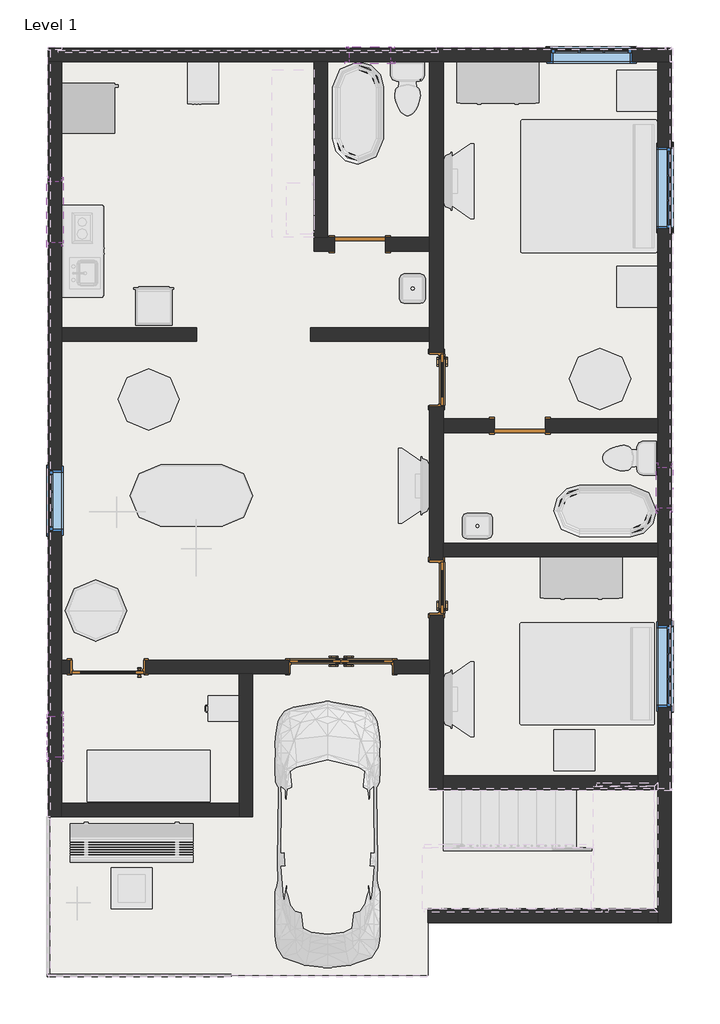
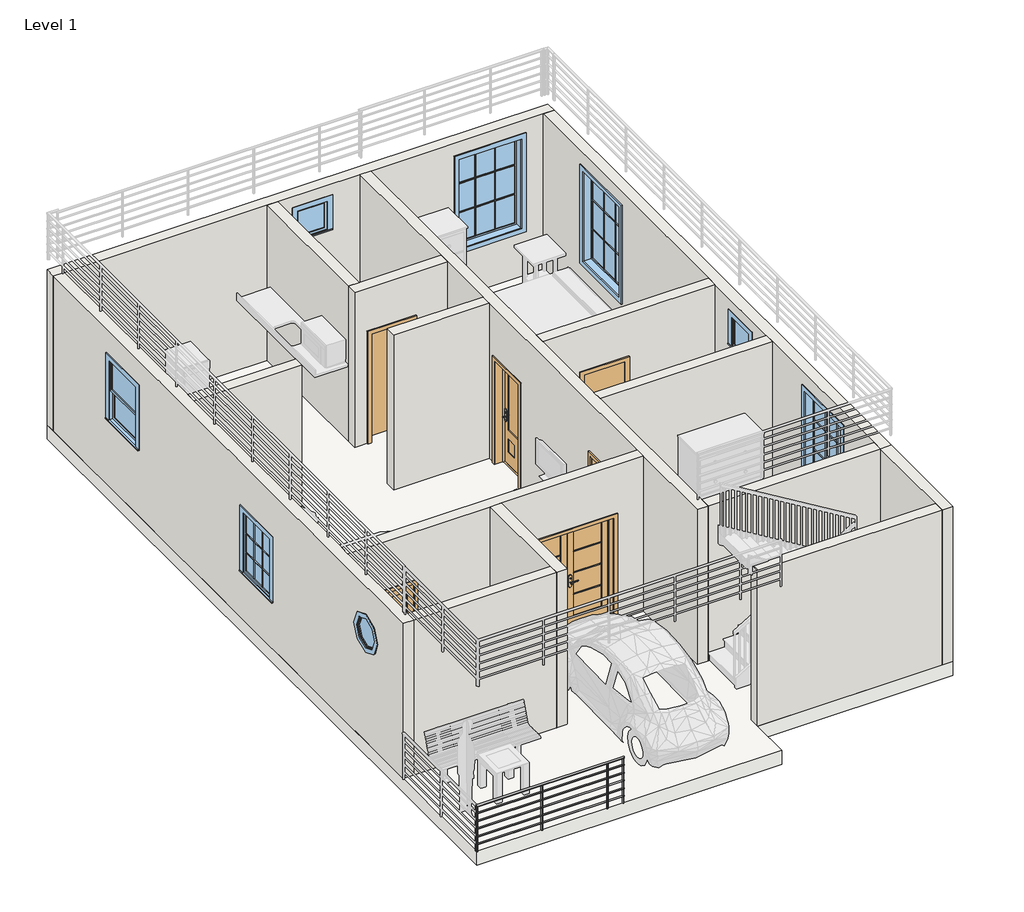
# One storey, part 1 of 4: 15 walls, 8 windows, 6 doors, 1 railing, 1 slab.
"""IFC4 building model written with IfcOpenShell, lengths in millimetres."""

from ifc_helpers import new_model, si_unit, point, frame, frame_2d, origin, origin_with_axes, place, context, project, spatial, polyline, circle_curve, trimmed, segment, composite_curve, outline, extrude, faceted_brep, transform, mapped, element, save
from ifc_brep_helpers import plane_surface, revolved_surface, advanced_brep
from components import door_ad59dcae, door_41326d50, door_b03bd389, door_f3911013, door_4314e8ec, window_29c06734, window_5a4e61ec, window_31198920, window_3923817a, window_e41d21a6

model = new_model("IFC4")

# Units and contexts
model_context = context("Model", 3, world=origin())
ifc_project = project(units=[si_unit("LENGTHUNIT", "METRE", prefix="MILLI")], contexts=[model_context])

# Site, building, storey
site = spatial("IfcSite", under=ifc_project)
building = spatial("IfcBuilding", under=site)
storey = spatial("IfcBuildingStorey", under=building, Name="Level 1", Elevation=0.0)

# Doors
placement = place(None, origin())
door_shape = door_ad59dcae(model_context)
element("IfcDoor", 1, ObjectType="30\" x 80\"", at=placement, inside=storey, context=model_context, shape_type="MappedRepresentation", body=[
    mapped(door_shape, transform((-8628.2639568, 7069.0342758, 0.0), x_axis=(0.0, -1.0, 0.0), y_axis=(1.0, 0.0, 0.0), z_axis=(0.0, 0.0, 1.0))),
])
door_2_shape = door_41326d50(model_context)
element("IfcDoor", 2, ObjectType="30\" x 80\"", at=placement, inside=storey, context=model_context, shape_type="MappedRepresentation", body=[
    mapped(door_2_shape, transform((-8628.2639568, 10167.8342758, 0.0), x_axis=(0.0, 1.0, 0.0), y_axis=(-1.0, 0.0, 0.0), z_axis=(0.0, 0.0, 1.0))),
])
door_3_shape = door_b03bd389(model_context)
element("IfcDoor", 3, ObjectType="Door-Exterior-Double-Full Glass-Wood_Clad : 60\" x 80\"", at=placement, inside=storey, context=model_context, shape_type="MappedRepresentation", body=[
    mapped(door_3_shape, transform((-10053.8389568, 5891.1092758, 0.0), x_axis=(1.0, 0.0, 0.0), y_axis=(0.0, 1.0, 0.0), z_axis=(0.0, 0.0, 1.0))),
])
door_4_shape = door_f3911013(model_context)
element("IfcDoor", 4, ObjectType="Door-Interior-Single-Full Glass-Wood : 42\" x 80\"", at=placement, inside=storey, context=model_context, shape_type="MappedRepresentation", body=[
    mapped(door_4_shape, transform((-13533.6389568, 5884.7592758, 0.0), x_axis=(-1.0, 0.0, 0.0), y_axis=(0.0, -1.0, 0.0), z_axis=(0.0, 0.0, 1.0))),
])
door_5_shape = door_4314e8ec(model_context)
element("IfcDoor", 5, ObjectType="Single-Flush : 30\" x 84\"", at=placement, inside=storey, context=model_context, shape_type="MappedRepresentation", body=[
    mapped(door_5_shape, transform((-9774.4389568, 12187.1342758, 0.0), x_axis=(-1.0, 0.0, 0.0), y_axis=(0.0, -1.0, 0.0), z_axis=(0.0, 0.0, 1.0))),
])
element("IfcDoor", 6, ObjectType="Single-Flush : 30\" x 84\"", at=placement, inside=storey, context=model_context, shape_type="MappedRepresentation", body=[
    mapped(door_5_shape, transform((-7386.8389568, 9482.0342758, 0.0), x_axis=(1.0, 0.0, 0.0), y_axis=(0.0, 1.0, 0.0), z_axis=(0.0, 0.0, 1.0))),
])

# Railing
element("IfcRailing", 7, ObjectType="Handrail - Pipe", at=placement, inside=storey, context=model_context, shape_type="SweptSolid", body=[
    extrude(outline(composite_curve([segment(trimmed(circle_curve(frame_2d((1290.5342758, 895.35)), 19.05), [point((1271.4842758, 895.35))], [point((1309.5842758, 895.35))], False, "CARTESIAN"), True, "CONTINUOUS"), segment(trimmed(circle_curve(frame_2d((1290.5342758, 895.35)), 19.05), [point((1309.5842758, 895.35))], [point((1271.4842758, 895.35))], False, "CARTESIAN"), True, "CONTINUOUS")], self_intersect=False)), frame((-14435.3389568, 0.0, 0.0), z_axis=(1.0, 0.0, 0.0), x_axis=(0.0, 1.0, 0.0)), (0.0, 0.0, 1.0), 2743.2),
    extrude(outline(composite_curve([segment(trimmed(circle_curve(frame_2d((1290.5342758, 749.3)), 12.7), [point((1303.2342758, 749.3))], [point((1277.8342758, 749.3))], False, "CARTESIAN"), True, "CONTINUOUS"), segment(trimmed(circle_curve(frame_2d((1290.5342758, 749.3)), 12.7), [point((1277.8342758, 749.3))], [point((1303.2342758, 749.3))], False, "CARTESIAN"), True, "CONTINUOUS")], self_intersect=False)), frame((-14435.3389568, 0.0, 0.0), z_axis=(1.0, 0.0, 0.0), x_axis=(0.0, 1.0, 0.0)), (0.0, 0.0, 1.0), 2743.2),
    extrude(outline(composite_curve([segment(trimmed(circle_curve(frame_2d((1290.5342758, 596.9)), 12.7), [point((1303.2342758, 596.9))], [point((1277.8342758, 596.9))], False, "CARTESIAN"), True, "CONTINUOUS"), segment(trimmed(circle_curve(frame_2d((1290.5342758, 596.9)), 12.7), [point((1277.8342758, 596.9))], [point((1303.2342758, 596.9))], False, "CARTESIAN"), True, "CONTINUOUS")], self_intersect=False)), frame((-14435.3389568, 0.0, 0.0), z_axis=(1.0, 0.0, 0.0), x_axis=(0.0, 1.0, 0.0)), (0.0, 0.0, 1.0), 2743.2),
    extrude(outline(composite_curve([segment(trimmed(circle_curve(frame_2d((1290.5342758, 444.5)), 12.7), [point((1303.2342758, 444.5))], [point((1277.8342758, 444.5))], False, "CARTESIAN"), True, "CONTINUOUS"), segment(trimmed(circle_curve(frame_2d((1290.5342758, 444.5)), 12.7), [point((1277.8342758, 444.5))], [point((1303.2342758, 444.5))], False, "CARTESIAN"), True, "CONTINUOUS")], self_intersect=False)), frame((-14435.3389568, 0.0, 0.0), z_axis=(1.0, 0.0, 0.0), x_axis=(0.0, 1.0, 0.0)), (0.0, 0.0, 1.0), 2743.2),
    extrude(outline(composite_curve([segment(trimmed(circle_curve(frame_2d((1290.5342758, 292.1)), 12.7), [point((1303.2342758, 292.1))], [point((1277.8342758, 292.1))], False, "CARTESIAN"), True, "CONTINUOUS"), segment(trimmed(circle_curve(frame_2d((1290.5342758, 292.1)), 12.7), [point((1277.8342758, 292.1))], [point((1303.2342758, 292.1))], False, "CARTESIAN"), True, "CONTINUOUS")], self_intersect=False)), frame((-14435.3389568, 0.0, 0.0), z_axis=(1.0, 0.0, 0.0), x_axis=(0.0, 1.0, 0.0)), (0.0, 0.0, 1.0), 2743.2),
    extrude(outline(composite_curve([segment(trimmed(circle_curve(frame_2d((1290.5342758, 139.7)), 12.7), [point((1303.2342758, 139.7))], [point((1277.8342758, 139.7))], False, "CARTESIAN"), True, "CONTINUOUS"), segment(trimmed(circle_curve(frame_2d((1290.5342758, 139.7)), 12.7), [point((1277.8342758, 139.7))], [point((1303.2342758, 139.7))], False, "CARTESIAN"), True, "CONTINUOUS")], self_intersect=False)), frame((-14435.3389568, 0.0, 0.0), z_axis=(1.0, 0.0, 0.0), x_axis=(0.0, 1.0, 0.0)), (0.0, 0.0, 1.0), 2743.2),
    extrude(outline(composite_curve([segment(trimmed(circle_curve(frame_2d((-11996.9389568, 1290.5342758)), 12.7), [point((-11996.9389568, 1303.2342758))], [point((-11996.9389568, 1277.8342758))], False, "CARTESIAN"), True, "CONTINUOUS"), segment(trimmed(circle_curve(frame_2d((-11996.9389568, 1290.5342758)), 12.7), [point((-11996.9389568, 1277.8342758))], [point((-11996.9389568, 1303.2342758))], False, "CARTESIAN"), True, "CONTINUOUS")], self_intersect=False)), origin_with_axes(), (0.0, 0.0, 1.0), 876.3),
    extrude(outline(composite_curve([segment(trimmed(circle_curve(frame_2d((-13216.1389568, 1290.5342758)), 12.7), [point((-13216.1389568, 1303.2342758))], [point((-13216.1389568, 1277.8342758))], False, "CARTESIAN"), True, "CONTINUOUS"), segment(trimmed(circle_curve(frame_2d((-13216.1389568, 1290.5342758)), 12.7), [point((-13216.1389568, 1277.8342758))], [point((-13216.1389568, 1303.2342758))], False, "CARTESIAN"), True, "CONTINUOUS")], self_intersect=False)), origin_with_axes(), (0.0, 0.0, 1.0), 876.3),
    extrude(outline(composite_curve([segment(trimmed(circle_curve(frame_2d((-11704.8389568, 1290.5342758)), 12.7), [point((-11704.8389568, 1303.2342758))], [point((-11704.8389568, 1277.8342758))], False, "CARTESIAN"), True, "CONTINUOUS"), segment(trimmed(circle_curve(frame_2d((-11704.8389568, 1290.5342758)), 12.7), [point((-11704.8389568, 1277.8342758))], [point((-11704.8389568, 1303.2342758))], False, "CARTESIAN"), True, "CONTINUOUS")], self_intersect=False)), origin_with_axes(), (0.0, 0.0, 1.0), 876.3),
    extrude(outline(composite_curve([segment(trimmed(circle_curve(frame_2d((-14422.6389568, 1290.5342758)), 12.7), [point((-14422.6389568, 1303.2342758))], [point((-14422.6389568, 1277.8342758))], False, "CARTESIAN"), True, "CONTINUOUS"), segment(trimmed(circle_curve(frame_2d((-14422.6389568, 1290.5342758)), 12.7), [point((-14422.6389568, 1277.8342758))], [point((-14422.6389568, 1303.2342758))], False, "CARTESIAN"), True, "CONTINUOUS")], self_intersect=False)), origin_with_axes(), (0.0, 0.0, 1.0), 876.3),
])

# Slab
element("IfcSlab", 8, ObjectType="Wood Joist 10\" - Ceramic Tile", at=placement, inside=storey, context=model_context, shape_type="SweptSolid", body=[
    extrude(outline(polyline([(-5126.2389568, 15108.1342758), (-5126.2389568, 2077.9342758), (-8758.4389568, 2077.9342758), (-8758.4389568, 1290.5342758), (-14422.6389568, 1290.5342758), (-14422.6389568, 15108.1342758), (-5126.2389568, 15108.1342758)])), frame((0.0, 0.0, -273.05), z_axis=(0.0, 0.0, 1.0), x_axis=(1.0, 0.0, 0.0)), (0.0, 0.0, 1.0), 273.05),
])

# Walls
element("IfcWall", 9, ObjectType="Generic - 8\"", at=placement, inside=storey, context=model_context, shape_type="Brep", body=[
    faceted_brep([(-14422.6389568, 14904.9342758, 0.0), (-14219.4389568, 14904.9342758, 0.0), (-10460.2389568, 14904.9342758, 0.0), (-10257.0389568, 14904.9342758, 0.0), (-8733.0389568, 14904.9342758, 0.0), (-8529.8389568, 14904.9342758, 0.0), (-5329.4389568, 14904.9342758, 0.0), (-5126.2389568, 14904.9342758, 0.0), (-5126.2389568, 14904.9342758, 3048.0), (-5329.4389568, 14904.9342758, 3048.0), (-8529.8389568, 14904.9342758, 3048.0), (-8733.0389568, 14904.9342758, 3048.0), (-10257.0389568, 14904.9342758, 3048.0), (-10460.2389568, 14904.9342758, 3048.0), (-14219.4389568, 14904.9342758, 3048.0), (-14422.6389568, 14904.9342758, 3048.0), (-5710.4389568, 14904.9342758, 2743.2), (-5710.4389568, 14904.9342758, 914.4), (-6929.6389568, 14904.9342758, 914.4), (-6929.6389568, 14904.9342758, 2743.2), (-9926.8389568, 14904.9342758, 2768.6), (-9317.2389568, 14904.9342758, 2768.6), (-9317.2389568, 14904.9342758, 2159.0), (-9926.8389568, 14904.9342758, 2159.0), (-14422.6389568, 15108.1342758, 0.0), (-14422.6389568, 15108.1342758, 3048.0), (-5126.2389568, 15108.1342758, 3048.0), (-5126.2389568, 15108.1342758, 0.0), (-5710.4389568, 15108.1342758, 2743.2), (-6929.6389568, 15108.1342758, 2743.2), (-6929.6389568, 15108.1342758, 914.4), (-5710.4389568, 15108.1342758, 914.4), (-9926.8389568, 15108.1342758, 2768.6), (-9926.8389568, 15108.1342758, 2159.0), (-9317.2389568, 15108.1342758, 2159.0), (-9317.2389568, 15108.1342758, 2768.6)], [[[0, 1, 2, 3, 4, 5, 6, 7, 8, 9, 10, 11, 12, 13, 14, 15], [16, 17, 18, 19], [20, 21, 22, 23]], [[24, 25, 26, 27], [28, 29, 30, 31], [32, 33, 34, 35]], [[7, 6, 5, 4, 3, 2, 1, 0, 24, 27]], [[8, 7, 27, 26]], [[0, 15, 25, 24]], [[15, 14, 13, 12, 11, 10, 9, 8, 26, 25]], [[17, 16, 28, 31]], [[18, 17, 31, 30]], [[19, 18, 30, 29]], [[16, 19, 29, 28]], [[33, 32, 20, 23]], [[34, 33, 23, 22]], [[35, 34, 22, 21]], [[32, 35, 21, 20]]]),
])
element("IfcWall", 10, ObjectType="Generic - 8\"", at=placement, inside=storey, context=model_context, shape_type="Brep", body=[
    faceted_brep([(-5329.4389568, 14904.9342758, 0.0), (-5329.4389568, 9583.6342758, 0.0), (-5329.4389568, 9380.4342758, 0.0), (-5329.4389568, 7729.4342758, 0.0), (-5329.4389568, 7526.2342758, 0.0), (-5329.4389568, 4262.3342758, 0.0), (-5329.4389568, 4059.1342758, 0.0), (-5329.4389568, 2281.1342758, 0.0), (-5329.4389568, 2077.9342758, 0.0), (-5329.4389568, 2077.9342758, 3048.0), (-5329.4389568, 2281.1342758, 3048.0), (-5329.4389568, 4059.1342758, 3048.0), (-5329.4389568, 4262.3342758, 3048.0), (-5329.4389568, 7526.2342758, 3048.0), (-5329.4389568, 7729.4342758, 3048.0), (-5329.4389568, 9380.4342758, 3048.0), (-5329.4389568, 9583.6342758, 3048.0), (-5329.4389568, 14904.9342758, 3048.0), (-5329.4389568, 12415.7342758, 2743.2), (-5329.4389568, 12415.7342758, 914.4), (-5329.4389568, 13634.9342758, 914.4), (-5329.4389568, 13634.9342758, 2743.2), (-5329.4389568, 5284.6842758, 2743.2), (-5329.4389568, 5284.6842758, 914.4), (-5329.4389568, 6503.8842758, 914.4), (-5329.4389568, 6503.8842758, 2743.2), (-5329.4389568, 8859.7342758, 2768.6), (-5329.4389568, 8250.1342758, 2768.6), (-5329.4389568, 8250.1342758, 2159.0), (-5329.4389568, 8859.7342758, 2159.0), (-5126.2389568, 14904.9342758, 0.0), (-5126.2389568, 14904.9342758, 3048.0), (-5126.2389568, 4059.1342758, 3048.0), (-5126.2389568, 2077.9342758, 3048.0), (-5126.2389568, 2077.9342758, 0.0), (-5126.2389568, 12415.7342758, 2743.2), (-5126.2389568, 13634.9342758, 2743.2), (-5126.2389568, 13634.9342758, 914.4), (-5126.2389568, 12415.7342758, 914.4), (-5126.2389568, 5284.6842758, 2743.2), (-5126.2389568, 6503.8842758, 2743.2), (-5126.2389568, 6503.8842758, 914.4), (-5126.2389568, 5284.6842758, 914.4), (-5126.2389568, 8859.7342758, 2768.6), (-5126.2389568, 8859.7342758, 2159.0), (-5126.2389568, 8250.1342758, 2159.0), (-5126.2389568, 8250.1342758, 2768.6)], [[[0, 1, 2, 3, 4, 5, 6, 7, 8, 9, 10, 11, 12, 13, 14, 15, 16, 17], [18, 19, 20, 21], [22, 23, 24, 25], [26, 27, 28, 29]], [[30, 31, 32, 33, 34], [35, 36, 37, 38], [39, 40, 41, 42], [43, 44, 45, 46]], [[8, 7, 6, 5, 4, 3, 2, 1, 0, 30, 34]], [[0, 17, 31, 30]], [[9, 8, 34, 33]], [[11, 10, 9, 33, 32]], [[17, 16, 15, 14, 13, 12, 11, 32, 31]], [[19, 18, 35, 38]], [[20, 19, 38, 37]], [[21, 20, 37, 36]], [[18, 21, 36, 35]], [[23, 22, 39, 42]], [[24, 23, 42, 41]], [[25, 24, 41, 40]], [[22, 25, 40, 39]], [[44, 43, 26, 29]], [[45, 44, 29, 28]], [[46, 45, 28, 27]], [[43, 46, 27, 26]]]),
])
element("IfcWall", 11, ObjectType="Generic - 8\"", at=placement, inside=storey, context=model_context, shape_type="Brep", body=[
    faceted_brep([(-8733.0389568, 14904.9342758, 3048.0), (-8733.0389568, 14904.9342758, 0.0), (-8733.0389568, 12288.7342758, 0.0), (-8733.0389568, 12085.5342758, 0.0), (-8733.0389568, 10942.5342758, 0.0), (-8733.0389568, 10739.3342758, 0.0), (-8733.0389568, 10574.2342758, 0.0), (-8733.0389568, 10574.2342758, 2057.4), (-8733.0389568, 9761.4342758, 2057.4), (-8733.0389568, 9761.4342758, 0.0), (-8733.0389568, 7475.4342758, 0.0), (-8733.0389568, 7475.4342758, 2057.4), (-8733.0389568, 6662.6342758, 2057.4), (-8733.0389568, 6662.6342758, 0.0), (-8733.0389568, 5989.5342758, 0.0), (-8733.0389568, 5786.3342758, 0.0), (-8733.0389568, 4059.1342758, 0.0), (-8733.0389568, 4059.1342758, 3048.0), (-8733.0389568, 5786.3342758, 3048.0), (-8733.0389568, 5989.5342758, 3048.0), (-8733.0389568, 10739.3342758, 3048.0), (-8733.0389568, 10942.5342758, 3048.0), (-8733.0389568, 12085.5342758, 3048.0), (-8733.0389568, 12288.7342758, 3048.0), (-8529.8389568, 14904.9342758, 0.0), (-8529.8389568, 14904.9342758, 3048.0), (-8529.8389568, 9583.6342758, 3048.0), (-8529.8389568, 9380.4342758, 3048.0), (-8529.8389568, 7729.4342758, 3048.0), (-8529.8389568, 7526.2342758, 3048.0), (-8529.8389568, 4262.3342758, 3048.0), (-8529.8389568, 4059.1342758, 3048.0), (-8529.8389568, 4059.1342758, 0.0), (-8529.8389568, 4262.3342758, 0.0), (-8529.8389568, 6662.6342758, 0.0), (-8529.8389568, 6662.6342758, 2057.4), (-8529.8389568, 7475.4342758, 2057.4), (-8529.8389568, 7475.4342758, 0.0), (-8529.8389568, 7526.2342758, 0.0), (-8529.8389568, 7729.4342758, 0.0), (-8529.8389568, 9380.4342758, 0.0), (-8529.8389568, 9583.6342758, 0.0), (-8529.8389568, 9761.4342758, 0.0), (-8529.8389568, 9761.4342758, 2057.4), (-8529.8389568, 10574.2342758, 2057.4), (-8529.8389568, 10574.2342758, 0.0)], [[[0, 1, 2, 3, 4, 5, 6, 7, 8, 9, 10, 11, 12, 13, 14, 15, 16, 17, 18, 19, 20, 21, 22, 23]], [[24, 25, 26, 27, 28, 29, 30, 31, 32, 33, 34, 35, 36, 37, 38, 39, 40, 41, 42, 43, 44, 45]], [[1, 24, 45, 6, 5, 4, 3, 2]], [[32, 16, 15, 14, 13, 34, 33]], [[37, 10, 9, 42, 41, 40, 39, 38]], [[1, 0, 25, 24]], [[17, 16, 32, 31]], [[12, 35, 34, 13]], [[35, 12, 11, 36]], [[36, 11, 10, 37]], [[44, 7, 6, 45]], [[7, 44, 43, 8]], [[8, 43, 42, 9]], [[0, 23, 22, 21, 20, 19, 18, 17, 31, 30, 29, 28, 27, 26, 25]]]),
])
element("IfcWall", 12, ObjectType="Generic - 8\"", at=placement, inside=storey, context=model_context, shape_type="Brep", body=[
    faceted_brep([(-10155.4389568, 12288.7342758, 2133.6), (-10155.4389568, 12288.7342758, 0.0), (-10257.0389568, 12288.7342758, 0.0), (-10460.2389568, 12288.7342758, 0.0), (-10460.2389568, 12288.7342758, 3048.0), (-10257.0389568, 12288.7342758, 3048.0), (-8733.0389568, 12288.7342758, 3048.0), (-8733.0389568, 12288.7342758, 0.0), (-9393.4389568, 12288.7342758, 0.0), (-9393.4389568, 12288.7342758, 2133.6), (-10460.2389568, 12085.5342758, 0.0), (-10155.4389568, 12085.5342758, 0.0), (-10155.4389568, 12085.5342758, 2133.6), (-9393.4389568, 12085.5342758, 2133.6), (-9393.4389568, 12085.5342758, 0.0), (-8733.0389568, 12085.5342758, 0.0), (-8733.0389568, 12085.5342758, 3048.0), (-10460.2389568, 12085.5342758, 3048.0)], [[[0, 1, 2, 3, 4, 5, 6, 7, 8, 9]], [[10, 11, 12, 13, 14, 15, 16, 17]], [[8, 7, 15, 14]], [[3, 2, 1, 11, 10]], [[4, 3, 10, 17]], [[7, 6, 16, 15]], [[12, 11, 1, 0]], [[13, 12, 0, 9]], [[14, 13, 9, 8]], [[6, 5, 4, 17, 16]]]),
])
element("IfcWall", 13, ObjectType="Generic - 8\"", at=placement, inside=storey, context=model_context, shape_type="SweptSolid", body=[
    extrude(outline(polyline([(-10511.0389568, 10942.5342758), (-8733.0389568, 10942.5342758), (-8733.0389568, 10739.3342758), (-10511.0389568, 10739.3342758), (-10511.0389568, 10942.5342758)])), origin_with_axes(), (0.0, 0.0, 1.0), 3048.0),
])
element("IfcWall", 14, ObjectType="Generic - 8\"", at=placement, inside=storey, context=model_context, shape_type="Brep", body=[
    faceted_brep([(-14219.4389568, 5989.5342758, 0.0), (-14219.4389568, 5989.5342758, 3048.0), (-8733.0389568, 5989.5342758, 3048.0), (-8733.0389568, 5989.5342758, 0.0), (-9266.4389568, 5989.5342758, 0.0), (-9266.4389568, 5989.5342758, 2057.4), (-10841.2389568, 5989.5342758, 2057.4), (-10841.2389568, 5989.5342758, 0.0), (-12974.8389568, 5989.5342758, 0.0), (-12974.8389568, 5989.5342758, 2057.4), (-14092.4389568, 5989.5342758, 2057.4), (-14092.4389568, 5989.5342758, 0.0), (-14219.4389568, 5786.3342758, 3048.0), (-14219.4389568, 5786.3342758, 0.0), (-14092.4389568, 5786.3342758, 0.0), (-14092.4389568, 5786.3342758, 2057.4), (-12974.8389568, 5786.3342758, 2057.4), (-12974.8389568, 5786.3342758, 0.0), (-11577.8389568, 5786.3342758, 0.0), (-11374.6389568, 5786.3342758, 0.0), (-10841.2389568, 5786.3342758, 0.0), (-10841.2389568, 5786.3342758, 2057.4), (-9266.4389568, 5786.3342758, 2057.4), (-9266.4389568, 5786.3342758, 0.0), (-8733.0389568, 5786.3342758, 0.0), (-8733.0389568, 5786.3342758, 3048.0), (-11374.6389568, 5786.3342758, 3048.0), (-11577.8389568, 5786.3342758, 3048.0)], [[[0, 1, 2, 3, 4, 5, 6, 7, 8, 9, 10, 11]], [[12, 13, 14, 15, 16, 17, 18, 19, 20, 21, 22, 23, 24, 25, 26, 27]], [[3, 24, 23, 4]], [[13, 0, 11, 14]], [[7, 20, 19, 18, 17, 8]], [[1, 0, 13, 12]], [[3, 2, 25, 24]], [[22, 5, 4, 23]], [[5, 22, 21, 6]], [[6, 21, 20, 7]], [[10, 15, 14, 11]], [[15, 10, 9, 16]], [[16, 9, 8, 17]], [[2, 1, 12, 27, 26, 25]]]),
])
element("IfcWall", 15, ObjectType="Generic - 8\"", at=placement, inside=storey, context=model_context, shape_type="Brep", body=[
    faceted_brep([(-11577.8389568, 5786.3342758, 0.0), (-11577.8389568, 3855.9342758, 0.0), (-11577.8389568, 3652.7342758, 0.0), (-11577.8389568, 3652.7342758, 3048.0), (-11577.8389568, 3855.9342758, 3048.0), (-11577.8389568, 5786.3342758, 3048.0), (-11374.6389568, 5786.3342758, 0.0), (-11374.6389568, 5786.3342758, 3048.0), (-11374.6389568, 3652.7342758, 3048.0), (-11374.6389568, 3652.7342758, 0.0)], [[[0, 1, 2, 3, 4, 5]], [[6, 7, 8, 9]], [[2, 1, 0, 6, 9]], [[0, 5, 7, 6]], [[3, 2, 9, 8]], [[5, 4, 3, 8, 7]]]),
])
element("IfcWall", 16, ObjectType="Generic - 8\"", at=placement, inside=storey, context=model_context, shape_type="SweptSolid", body=[
    extrude(outline(polyline([(-14219.4389568, 3855.9342758), (-11577.8389568, 3855.9342758), (-11577.8389568, 3652.7342758), (-14219.4389568, 3652.7342758), (-14219.4389568, 3855.9342758)])), origin_with_axes(), (0.0, 0.0, 1.0), 3048.0),
])
element("IfcWall", 17, ObjectType="Generic - 8\"", at=placement, inside=storey, context=model_context, shape_type="SweptSolid", body=[
    extrude(outline(polyline([(-5329.4389568, 4059.1342758), (-8529.8389568, 4059.1342758), (-8529.8389568, 4262.3342758), (-5329.4389568, 4262.3342758), (-5329.4389568, 4059.1342758)])), origin_with_axes(), (0.0, 0.0, 1.0), 3048.0),
])
element("IfcWall", 18, ObjectType="Generic - 8\"", at=placement, inside=storey, context=model_context, shape_type="SweptSolid", body=[
    extrude(outline(polyline([(-5329.4389568, 7526.2342758), (-8529.8389568, 7526.2342758), (-8529.8389568, 7729.4342758), (-5329.4389568, 7729.4342758), (-5329.4389568, 7526.2342758)])), origin_with_axes(), (0.0, 0.0, 1.0), 3048.0),
])
element("IfcWall", 19, ObjectType="Generic - 8\"", at=placement, inside=storey, context=model_context, shape_type="SweptSolid", body=[
    extrude(outline(polyline([(2133.6, -7005.8389568), (0.0, -7005.8389568), (0.0, -5329.4389568), (3048.0, -5329.4389568), (3048.0, -8529.8389568), (0.0, -8529.8389568), (0.0, -7767.8389568), (2133.6, -7767.8389568), (2133.6, -7005.8389568)])), frame((0.0, 9380.4342758, 0.0), z_axis=(0.0, 1.0, 0.0), x_axis=(0.0, 0.0, 1.0)), (0.0, 0.0, 1.0), 203.2),
])
element("IfcWall", 20, ObjectType="Generic - 8\"", at=placement, inside=storey, context=model_context, shape_type="AdvancedBrep", body=[
    advanced_brep(
    [(-14219.4389568, 3652.7342758, 0.0), (-14219.4389568, 3855.9342758, 0.0), (-14219.4389568, 5786.3342758, 0.0), (-14219.4389568, 5989.5342758, 0.0), (-14219.4389568, 10739.3342758, 0.0), (-14219.4389568, 10942.5342758, 0.0), (-14219.4389568, 14904.9342758, 0.0), (-14219.4389568, 14904.9342758, 3048.0), (-14219.4389568, 10942.5342758, 3048.0), (-14219.4389568, 10739.3342758, 3048.0), (-14219.4389568, 5989.5342758, 3048.0), (-14219.4389568, 5786.3342758, 3048.0), (-14219.4389568, 3855.9342758, 3048.0), (-14219.4389568, 3652.7342758, 3048.0), (-14219.4389568, 8821.6342758, 2133.6), (-14219.4389568, 8821.6342758, 914.4), (-14219.4389568, 7907.2342758, 914.4), (-14219.4389568, 7907.2342758, 2133.6), (-14219.4389568, 13126.9342758, 2514.6), (-14219.4389568, 13126.9342758, 1295.4), (-14219.4389568, 12212.5342758, 1295.4), (-14219.4389568, 12212.5342758, 2514.6), (-14219.4389568, 4541.7342758, 2133.6), (-14219.4389568, 5151.3342758, 2133.6), (-14422.6389568, 3652.7342758, 0.0), (-14422.6389568, 3652.7342758, 3048.0), (-14422.6389568, 14904.9342758, 3048.0), (-14422.6389568, 14904.9342758, 0.0), (-14422.6389568, 8821.6342758, 2133.6), (-14422.6389568, 7907.2342758, 2133.6), (-14422.6389568, 7907.2342758, 914.4), (-14422.6389568, 8821.6342758, 914.4), (-14422.6389568, 13126.9342758, 2514.6), (-14422.6389568, 12212.5342758, 2514.6), (-14422.6389568, 12212.5342758, 1295.4), (-14422.6389568, 13126.9342758, 1295.4), (-14422.6389568, 4541.7342758, 2133.6), (-14422.6389568, 5151.3342758, 2133.6)],
    [
        (0, 1),
        (1, 2),
        (2, 3),
        (3, 4),
        (4, 5),
        (5, 6),
        (6, 7),
        (7, 8),
        (8, 9),
        (9, 10),
        (10, 11),
        (11, 12),
        (12, 13),
        (13, 0),
        (14, 15),
        (15, 16),
        (16, 17),
        (17, 14),
        (18, 19),
        (19, 20),
        (20, 21),
        (21, 18),
        (22, 23, circle_curve(frame((-14219.4389568, 4846.5342758, 2133.6), z_axis=(-1.0, 0.0, 0.0), x_axis=(0.0, 1.0, 0.0)), 304.8)),
        (23, 22, circle_curve(frame((-14219.4389568, 4846.5342758, 2133.6), z_axis=(-1.0, 0.0, 0.0), x_axis=(0.0, 1.0, 0.0)), 304.8)),
        (24, 25),
        (25, 26),
        (26, 27),
        (27, 24),
        (28, 29),
        (29, 30),
        (30, 31),
        (31, 28),
        (32, 33),
        (33, 34),
        (34, 35),
        (35, 32),
        (36, 37, circle_curve(frame((-14422.6389568, 4846.5342758, 2133.6), z_axis=(1.0, 0.0, 0.0), x_axis=(0.0, 1.0, 0.0)), 304.8)),
        (37, 36, circle_curve(frame((-14422.6389568, 4846.5342758, 2133.6), z_axis=(1.0, 0.0, 0.0), x_axis=(0.0, 1.0, 0.0)), 304.8)),
        (0, 24),
        (27, 6),
        (26, 7),
        (13, 25),
        (14, 28),
        (31, 15),
        (30, 16),
        (29, 17),
        (18, 32),
        (35, 19),
        (34, 20),
        (33, 21),
        (36, 22),
        (23, 37),
    ],
    [
        plane_surface(frame((-14219.4389568, 1315.9342758, 0.0), z_axis=(1.0, 0.0, 0.0), x_axis=(0.0, 1.0, 0.0))),
        plane_surface(frame((-14422.6389568, 1315.9342758, 0.0), z_axis=(-1.0, 0.0, 0.0), x_axis=(0.0, -1.0, 0.0))),
        plane_surface(frame((-14219.4389568, 3754.3342758, 0.0), z_axis=(0.0, 0.0, -1.0), x_axis=(-1.0, 0.0, 0.0))),
        plane_surface(frame((-14321.0389568, 14904.9342758, 0.0), z_axis=(0.0, 1.0, 0.0), x_axis=(1.0, 0.0, 0.0))),
        plane_surface(frame((-11476.2389568, 3652.7342758, 0.0), z_axis=(0.0, -1.0, 0.0), x_axis=(1.0, 0.0, 0.0))),
        plane_surface(frame((-14422.6389568, 15108.1342758, 3048.0), z_axis=(0.0, 0.0, 1.0), x_axis=(1.0, 0.0, 0.0))),
        plane_surface(frame((-14219.4389568, 8821.6342758, 2133.6), z_axis=(0.0, -1.0, 0.0), x_axis=(-1.0, 0.0, 0.0))),
        plane_surface(frame((-14219.4389568, 8821.6342758, 914.4), z_axis=(0.0, 0.0, 1.0), x_axis=(-1.0, 0.0, 0.0))),
        plane_surface(frame((-14219.4389568, 7907.2342758, 914.4), z_axis=(0.0, 1.0, 0.0), x_axis=(-1.0, 0.0, 0.0))),
        plane_surface(frame((-14219.4389568, 7907.2342758, 2133.6), z_axis=(0.0, 0.0, -1.0), x_axis=(-1.0, 0.0, 0.0))),
        plane_surface(frame((-14219.4389568, 13126.9342758, 2514.6), z_axis=(0.0, -1.0, 0.0), x_axis=(-1.0, 0.0, 0.0))),
        plane_surface(frame((-14219.4389568, 13126.9342758, 1295.4), z_axis=(0.0, 0.0, 1.0), x_axis=(-1.0, 0.0, 0.0))),
        plane_surface(frame((-14219.4389568, 12212.5342758, 1295.4), z_axis=(0.0, 1.0, 0.0), x_axis=(-1.0, 0.0, 0.0))),
        plane_surface(frame((-14219.4389568, 12212.5342758, 2514.6), z_axis=(0.0, 0.0, -1.0), x_axis=(-1.0, 0.0, 0.0))),
        revolved_surface(polyline([(-14219.4389568, 5151.3342758, 2133.6), (-14422.6389568, 5151.3342758, 2133.6)]), (-14219.4389568, 4846.5342758, 2133.6), (1.0, 0.0, 0.0)),
    ],
    [
        (0, [[1, 2, 3, 4, 5, 6, 7, 8, 9, 10, 11, 12, 13, 14], [15, 16, 17, 18], [19, 20, 21, 22], [23, 24]]),
        (1, [[25, 26, 27, 28], [29, 30, 31, 32], [33, 34, 35, 36], [37, 38]]),
        (2, [[-6, -5, -4, -3, -2, -1, 39, -28, 40]]),
        (3, [[-7, -40, -27, 41]]),
        (4, [[-14, 42, -25, -39]]),
        (5, [[-13, -12, -11, -10, -9, -8, -41, -26, -42]]),
        (6, [[-15, 43, -32, 44]]),
        (7, [[-16, -44, -31, 45]]),
        (8, [[-17, -45, -30, 46]]),
        (9, [[-18, -46, -29, -43]]),
        (10, [[-19, 47, -36, 48]]),
        (11, [[-20, -48, -35, 49]]),
        (12, [[-21, -49, -34, 50]]),
        (13, [[-22, -50, -33, -47]]),
        (14, [[-37, 51, -24, 52]]),
        (14, [[-38, -52, -23, -51]]),
    ],
),
])
element("IfcWall", 21, ObjectType="Generic - 8\"", at=placement, inside=storey, context=model_context, shape_type="SweptSolid", body=[
    extrude(outline(polyline([(0.0, -5329.4389568), (3048.0, -5329.4389568), (3048.0, -8733.0389568), (3048.0, -8758.4389568), (0.0, -8758.4389568), (0.0, -5329.4389568)])), frame((0.0, 2077.9342758, 0.0), z_axis=(0.0, 1.0, 0.0), x_axis=(0.0, 0.0, 1.0)), (0.0, 0.0, 1.0), 203.2),
])
element("IfcWall", 22, ObjectType="Generic - 8\"", at=placement, inside=storey, context=model_context, shape_type="SweptSolid", body=[
    extrude(outline(polyline([(-10460.2389568, 12288.7342758), (-10460.2389568, 14904.9342758), (-10257.0389568, 14904.9342758), (-10257.0389568, 12288.7342758), (-10460.2389568, 12288.7342758)])), origin_with_axes(), (0.0, 0.0, 1.0), 3048.0),
])
element("IfcWall", 23, ObjectType="Generic - 8\"", at=placement, inside=storey, context=model_context, shape_type="SweptSolid", body=[
    extrude(outline(polyline([(-14219.4389568, 10942.5342758), (-12212.8389568, 10942.5342758), (-12212.8389568, 10739.3342758), (-14219.4389568, 10739.3342758), (-14219.4389568, 10942.5342758)])), origin_with_axes(), (0.0, 0.0, 1.0), 3048.0),
])

# Windows
window_shape = window_29c06734(model_context)
element("IfcWindow", 24, ObjectType="Casement 3x3 with Trim : 36\" x 48\"", at=placement, inside=storey, context=model_context, shape_type="MappedRepresentation", body=[
    mapped(window_shape, transform((-14321.0389568, 8364.4342758, 0.0), x_axis=(0.0, 1.0, 0.0), y_axis=(-1.0, 0.0, 0.0), z_axis=(0.0, 0.0, 1.0))),
])
window_2_shape = window_5a4e61ec(model_context)
element("IfcWindow", 25, ObjectType="Casement 3x3 with Trim : 48\" x 72\"", at=placement, inside=storey, context=model_context, shape_type="MappedRepresentation", body=[
    mapped(window_2_shape, transform((-6320.0389568, 15006.5342758, 609.6), x_axis=(1.0, 0.0, 0.0), y_axis=(0.0, 1.0, 0.0), z_axis=(0.0, 0.0, 1.0))),
])
element("IfcWindow", 26, ObjectType="Casement 3x3 with Trim : 48\" x 72\"", at=placement, inside=storey, context=model_context, shape_type="MappedRepresentation", body=[
    mapped(window_2_shape, transform((-5227.8389568, 13025.3342758, 609.6), x_axis=(0.0, -1.0, 0.0), y_axis=(1.0, 0.0, 0.0), z_axis=(0.0, 0.0, 1.0))),
])
element("IfcWindow", 27, ObjectType="Casement 3x3 with Trim : 48\" x 72\"", at=placement, inside=storey, context=model_context, shape_type="MappedRepresentation", body=[
    mapped(window_2_shape, transform((-5227.8389568, 5894.2842758, 609.6), x_axis=(0.0, -1.0, 0.0), y_axis=(1.0, 0.0, 0.0), z_axis=(0.0, 0.0, 1.0))),
])
window_3_shape = window_31198920(model_context)
element("IfcWindow", 28, ObjectType="Double Hung with Trim : 36\" x 48\"", at=placement, inside=storey, context=model_context, shape_type="MappedRepresentation", body=[
    mapped(window_3_shape, transform((-14321.0389568, 12669.7342758, 381.0), x_axis=(0.0, 1.0, 0.0), y_axis=(-1.0, 0.0, 0.0), z_axis=(0.0, 0.0, 1.0))),
])
window_4_shape = window_3923817a(model_context)
element("IfcWindow", 29, ObjectType="Round with Trim : 48\" Diameter", at=placement, inside=storey, context=model_context, shape_type="MappedRepresentation", body=[
    mapped(window_4_shape, transform((-14321.0389568, 4998.9342758, 1219.2), x_axis=(0.0, 1.0, 0.0), y_axis=(-1.0, 0.0, 0.0), z_axis=(0.0, 0.0, 1.0))),
])
window_5_shape = window_e41d21a6(model_context)
element("IfcWindow", 30, ObjectType="Transom with Trim : 24\" x 24\"", at=placement, inside=storey, context=model_context, shape_type="MappedRepresentation", body=[
    mapped(window_5_shape, transform((-9660.1389568, 15006.5342758, 0.0), x_axis=(-1.0, 0.0, 0.0), y_axis=(0.0, -1.0, 0.0), z_axis=(0.0, 0.0, 1.0))),
])
element("IfcWindow", 31, ObjectType="Transom with Trim : 24\" x 24\"", at=placement, inside=storey, context=model_context, shape_type="MappedRepresentation", body=[
    mapped(window_5_shape, transform((-5227.8389568, 8593.0342758, 0.0), x_axis=(0.0, 1.0, 0.0), y_axis=(-1.0, 0.0, 0.0), z_axis=(0.0, 0.0, 1.0))),
])

save(model, "model.ifc")

# Revit data of these elements
# Type "30\" x 80\""
#   Type Mark = "9"
#   Assembly Code = "B2030100"
#   Analytic Construction = "French door, wood frame with single glass"
#   Threshold Offset [instance default] = 0' - 0 1/2"
#   Thickness = 0' - 1 3/8"
#   Thermal Resistance (R) = 1.0696 (h·ft²·°F)/BTU
#   Swing Angle [instance default] = 90.00°
#   Stiles = 0' - 4 3/4"
#   Rough Width = 2' - 8"
#   Rough Height = 6' - 9"
#   Radius = 1' - 1.00625"
#   Lock Rail = 0' - 7 1/8"
#   Height = 6' - 8"
#   Width = 2' - 6"
#   Heat Transfer Coefficient (U) = 0.9350 BTU/(h·ft²·°F)
#   Door Offset [instance default] = 0' - 0"
#   Bottom Rail = 0' - 9 1/2"
#   Threshold [instance default] = yes
#   Function = 1
#   Exterior Trim [instance default] = yes
#   Trim Material = Cherry
#   Threshold Material = Cherry
#   Panel Material = Cherry
#   Glazing = Glass
#   Frame Material = Cherry
#   Door Handle Material = Aluminum
#   Visual Light Transmittance = 0
#   Solar Heat Gain Coefficient = 0
#   Wall Closure = (empty or 0)
#   Construction Type = (empty or 0)
# Type "Door-Exterior-Double-Full Glass-Wood_Clad : 60\" x 80\""
#   Type Mark = "8"
#   Assembly Code = "B2030100"
#   Analytic Construction = "French door, wood frame with double glass"
#   Top Rail = 0' - 4 11/16"
#   Threshold Offset [instance default] = 0' - 0 1/2"
#   Thickness = 0' - 1 3/8"
#   Thermal Resistance (R) = 1.9158 (h·ft²·°F)/BTU
#   Swing Angle [instance default] = 90.00°
#   Stiles = 0' - 4 3/4"
#   Rough Width = 5' - 2"
#   Rough Height = 6' - 9"
#   Panel Width = 2' - 6"
#   Door Offset [instance default] = 0' - 0"
#   Height = 6' - 8"
#   Width = 5' - 0"
#   Heat Transfer Coefficient (U) = 0.5220 BTU/(h·ft²·°F)
#   Bottom Rail = 0' - 9 1/8"
#   Exterior Trim [instance default] = yes
#   Threshold [instance default] = yes
#   Show Grill [instance default] = yes
#   Function = 1
#   Trim Material = Cherry
#   Threshold Material = Cherry
#   Panel Material = Cherry
#   Glazing = Glass
#   Frame Material = Cherry
#   Door Handle Material = Aluminum
#   Visual Light Transmittance = 0
#   Solar Heat Gain Coefficient = 0
#   Wall Closure = (empty or 0)
#   Construction Type = (empty or 0)
# Type "Door-Interior-Single-Full Glass-Wood : 42\" x 80\""
#   Type Mark = "10"
#   Assembly Code = "C1020300"
#   Analytic Construction = "Wood frame with single clear glass"
#   Top Rail = 0' - 4 11/16"
#   Thickness = 0' - 1 3/8"
#   Thermal Resistance (R) = 1.0102 (h·ft²·°F)/BTU
#   Swing Angle [instance default] = 90.00°
#   Stiles = 0' - 4 3/4"
#   Rough Width = 3' - 8"
#   Rough Height = 6' - 9"
#   Height = 6' - 8"
#   Width = 3' - 6"
#   Heat Transfer Coefficient (U) = 0.9900 BTU/(h·ft²·°F)
#   Bottom Rail = 0' - 9 1/8"
#   Show Grill [instance default] = yes
#   Trim Material = Cherry
#   Panel Material = Cherry
#   Frame Material = Cherry
#   Door Handle Material = Aluminum
#   Visual Light Transmittance = 0
#   Solar Heat Gain Coefficient = 0
#   Wall Closure = (empty or 0)
#   Function = (empty or 0)
# Type "Single-Flush : 30\" x 84\""
#   Type Mark = "4"
#   Construction Type Id = "MDOOR"
#   Assembly Code = "C1020"
#   Analytic Construction = "Metal"
#   Thickness = 0' - 2"
#   Heat Transfer Coefficient (U) = 0.651978 BTU/(h·ft²·°F)
#   Height = 7' - 0"
#   Trim Projection Ext = 0' - 1"
#   Trim Projection Int = 0' - 1"
#   Trim Width = 0' - 3"
#   Width = 2' - 6"
#   Define Thermal Properties by = 1
#   Door Material = Door - Panel
#   Frame Material = Door - Frame
#   Visual Light Transmittance = 0
#   Solar Heat Gain Coefficient = 0
#   Function = (empty or 0)
#   Wall Closure = (empty or 0)
# Type "Handrail - Pipe"
#   Assembly Code = "C2010400"
#   built-in parameter 1008612 = 0.0416667 (stored number, unit not read)
#   built-in parameter 1008611 = 0.0833333 (stored number, unit not read)
#   built-in parameter 1008609 = 4 (stored number, unit not read)
#   built-in parameter 1008604 = 0.166667 (stored number, unit not read)
#   built-in parameter 1008603 = 0.166667 (stored number, unit not read)
#   Railing Height = 3' - 0"
#   built-in parameter 1008630 = 2
#   built-in parameter 1008610 = 1
#   built-in parameter 1008605 = 1
#   built-in parameter 1008618 = Baluster - Round : 1"
# Type "Wood Joist 10\" - Ceramic Tile"
#   Assembly Code = "B1010"
#   Function = 0
#   Layers, outside or top first: 0' - 0 1/4" "Tile, Mosaic, Gray" (function 5); 0' - 0 1/2" "Concrete, Cast-in-Place gray" (function 4); 0' - 0 3/4" "Plywood, Sheathing" (function 1); 0' - 9 1/4" "Structure, Wood Joist/Rafter Layer" (function 1)
# Type "Generic - 8\""
#   Assembly Code = "B2010"
#   Layers, outside or top first: 0' - 8" "Brick, Common" (function 1)
# Type "Casement 3x3 with Trim : 36\" x 48\""
#   Type Mark = "10"
#   Construction Type Id = "GSP4R"
#   Assembly Code = "B2020100"
#   Analytic Construction = "1/8 in Pilkington single glazing"
#   Visual Light Transmittance = 0.9
#   Solar Heat Gain Coefficient = 0.78
#   Heat Transfer Coefficient (U) = 0.6496 BTU/(h·ft²·°F)
#   Height = 4' - 0"
#   Default Sill Height = 3' - 0"
#   Trim Projection - Ext. = 0' - 0 1/2"
#   Trim Projection - Int. = 0' - 0 3/4"
#   Trim Width - Exterior = 0' - 3 1/2"
#   Trim Width - Interior = 0' - 3 1/2"
#   Width = 3' - 0"
#   Window Inset = 0' - 0 3/4"
#   Define Thermal Properties by = 1
#   Glass Pane Material = Glass
#   Sash Material = Sash
#   Trim Exterior Material = Trim
#   Trim Interior Material = Trim
#   Wall Closure = (empty or 0)
# Type "Casement 3x3 with Trim : 48\" x 72\""
#   Type Mark = "12"
#   Construction Type Id = "GSP4R"
#   Assembly Code = "B2020100"
#   Analytic Construction = "1/8 in Pilkington single glazing"
#   Visual Light Transmittance = 0.9
#   Solar Heat Gain Coefficient = 0.78
#   Heat Transfer Coefficient (U) = 0.6496 BTU/(h·ft²·°F)
#   Height = 6' - 0"
#   Default Sill Height = 1' - 0"
#   Trim Projection - Ext. = 0' - 0 1/2"
#   Trim Projection - Int. = 0' - 0 3/4"
#   Trim Width - Exterior = 0' - 3 1/2"
#   Trim Width - Interior = 0' - 3 1/2"
#   Width = 4' - 0"
#   Window Inset = 0' - 0 3/4"
#   Define Thermal Properties by = 1
#   Glass Pane Material = Glass
#   Sash Material = Sash
#   Trim Exterior Material = Trim
#   Trim Interior Material = Trim
#   Wall Closure = (empty or 0)
# Type "Double Hung with Trim : 36\" x 48\""
#   Type Mark = "13"
#   Construction Type Id = "GSP4R"
#   Assembly Code = "B2020100"
#   Analytic Construction = "1/8 in Pilkington single glazing"
#   Visual Light Transmittance = 0.9
#   Solar Heat Gain Coefficient = 0.78
#   Heat Transfer Coefficient (U) = 0.6496 BTU/(h·ft²·°F)
#   Height = 4' - 0"
#   Default Sill Height = 3' - 0"
#   Trim Projection - Ext. = 0' - 0 1/2"
#   Trim Projection - Int. = 0' - 0 3/4"
#   Trim Width - Exterior = 0' - 3 1/2"
#   Trim Width - Interior = 0' - 3 1/2"
#   Width = 3' - 0"
#   Window Inset = 0' - 0 3/4"
#   Define Thermal Properties by = 1
#   Glass Pane Material = Glass
#   Sash Material = Sash
#   Trim Exterior Material = Trim
#   Trim Interior Material = Trim
#   Wall Closure = (empty or 0)
# Type "Round with Trim : 48\" Diameter"
#   Type Mark = "32"
#   Construction Type Id = "GSP4R"
#   Assembly Code = "B2020100"
#   Analytic Construction = "1/8 in Pilkington single glazing"
#   Visual Light Transmittance = 0.9
#   Solar Heat Gain Coefficient = 0.78
#   Heat Transfer Coefficient (U) = 0.6496 BTU/(h·ft²·°F)
#   Default Sill Height = 2' - 0"
#   Trim Projection - Ext. = 0' - 0 1/2"
#   Trim Projection - Int. = 0' - 0 3/4"
#   Trim Width - Exterior = 0' - 3 1/2"
#   Trim Width - Interior = 0' - 3 1/2"
#   Width = 2' - 0"
#   Define Thermal Properties by = 1
#   Glass Pane Material = Glass
#   Sash Material = Sash
#   Trim Exterior Material = Trim
#   Trim Interior Material = Trim
#   Wall Closure = (empty or 0)
# Type "Transom with Trim : 24\" x 24\""
#   Type Mark = "22"
#   Construction Type Id = "GSP4R"
#   Assembly Code = "B2020100"
#   Analytic Construction = "1/8 in Pilkington single glazing"
#   Visual Light Transmittance = 0.9
#   Solar Heat Gain Coefficient = 0.78
#   Heat Transfer Coefficient (U) = 0.6496 BTU/(h·ft²·°F)
#   Height = 2' - 0"
#   Default Sill Height = 7' - 1"
#   Trim Projection - Ext. = 0' - 0 1/2"
#   Trim Projection - Int. = 0' - 0 3/4"
#   Trim Width - Exterior = 0' - 3 1/2"
#   Trim Width - Interior = 0' - 3 1/2"
#   Width = 2' - 0"
#   Window Inset = 0' - 0 3/4"
#   Define Thermal Properties by = 1
#   Glass Pane Material = Glass
#   Sash Material = Sash
#   Trim Exterior Material = Trim
#   Trim Interior Material = Trim
#   Wall Closure = (empty or 0)
# Elements 1, 2 (IfcDoor, "30\" x 80\"")
#   Threshold Offset = 0' - 0 1/2"
#   Swing Angle = 90.00°
#   Door Offset = 0' - 0"
#   Threshold = yes
#   Exterior Trim = yes
#   Phase Created = New Construction
#   Materials on its faces: "Cherry", "Aluminum", "Glass"
# Element 3 (IfcDoor, "Door-Exterior-Double-Full Glass-Wood_Clad : 60\" x 80\"")
#   Threshold Offset = 0' - 0 1/2"
#   Swing Angle = 90.00°
#   Door Offset = 0' - 0"
#   Threshold = yes
#   Show Grill = yes
#   Exterior Trim = yes
#   Phase Created = New Construction
#   Materials on its faces: "Cherry", "Aluminum", "Glass"
# Element 4 (IfcDoor, "Door-Interior-Single-Full Glass-Wood : 42\" x 80\"")
#   Swing Angle = 90.00°
#   Show Grill = yes
#   Phase Created = New Construction
#   Materials on its faces: "Cherry", "Aluminum", "Glass"
# Elements 5, 6 (IfcDoor, "Single-Flush : 30\" x 84\"")
#   Phase Created = New Construction
#   Materials on its faces: "Door - Frame", "Door - Panel"
# Element 7 (IfcRailing, "Handrail - Pipe")
#   Phase Created = New Construction
# Element 8 (IfcSlab, "Wood Joist 10\" - Ceramic Tile")
#   Height Offset From Level = 0' - 0"
#   Phase Created = New Construction
#   Materials on its faces: "Structure, Wood Joist/Rafter Layer", "Tile, Mosaic, Gray"
# Elements 9, 10, 11, 12, 13, 14, 15, 16, 17, 18, 19, 20, 21, 22, 23 (IfcWall, "Generic - 8\"")
#   Top Offset = 0' - 0"
#   Base Offset = 0' - 0"
#   Unconnected Height = 10' - 0"
#   wall height = 10' - 0"
#   Phase Created = New Construction
#   Base Constraint = Level 1
#   Materials on its faces: "Brick, Common"
# Element 24 (IfcWindow, "Casement 3x3 with Trim : 36\" x 48\"")
#   Mark = "1"
#   Phase Created = New Construction
#   Materials on its faces: "Sash", "Glass", "Trim"
# Element 25 (IfcWindow, "Casement 3x3 with Trim : 48\" x 72\"")
#   Mark = "2"
#   Phase Created = New Construction
#   Materials on its faces: "Sash", "Glass", "Trim"
# Element 26 (IfcWindow, "Casement 3x3 with Trim : 48\" x 72\"")
#   Mark = "3"
#   Phase Created = New Construction
#   Materials on its faces: "Sash", "Glass", "Trim"
# Element 27 (IfcWindow, "Casement 3x3 with Trim : 48\" x 72\"")
#   Mark = "4"
#   Phase Created = New Construction
#   Materials on its faces: "Sash", "Glass", "Trim"
# Element 28 (IfcWindow, "Double Hung with Trim : 36\" x 48\"")
#   Mark = "5"
#   Phase Created = New Construction
#   Materials on its faces: "Sash", "Trim", "Glass"
# Element 29 (IfcWindow, "Round with Trim : 48\" Diameter")
#   Mark = "8"
#   Phase Created = New Construction
#   Materials on its faces: "Trim", "Sash", "Glass"
# Element 30 (IfcWindow, "Transom with Trim : 24\" x 24\"")
#   Mark = "6"
#   Phase Created = New Construction
#   Materials on its faces: "Sash", "Trim", "Glass"
# Element 31 (IfcWindow, "Transom with Trim : 24\" x 24\"")
#   Mark = "7"
#   Phase Created = New Construction
#   Materials on its faces: "Sash", "Trim", "Glass"
# Materials
#   "Cherry": class "Wood", colour RGB 226 177 128, transparency 0, Description = "Prunus Serotina", Cost = 0
#   "Glass": class "Glass", colour RGB 0 128 192, transparency 0.75, Description = "Soda Lime Glass", Cost = 0
#   "Aluminum": class "Metal", colour RGB 247 247 247, transparency 0, Description = "Aluminum 6061", Cost = 0
#   "Door - Panel": class "Wood", colour RGB 210 159 95, transparency 0
#   "Door - Frame": colour RGB 118 70 51, transparency 0
#   "Tile, Mosaic, Gray": class "Generic", colour RGB 127 127 127, transparency 0, Description = "Mosiac tile, gray", Cost = 0
#   "Concrete, Cast-in-Place gray": class "Concrete", colour RGB 192 192 192, transparency 0, Description = "Cast-in-place concrete", Cost = 0
#   "Plywood, Sheathing": class "Wood", colour RGB 212 179 113, transparency 0, Description = "Plywood, sheathing grade", Cost = 0
#   "Structure, Wood Joist/Rafter Layer": class "Wood", colour RGB 127 127 127, transparency 0, Description = "Wood framing, thermal airspace", Cost = 0
#   "Brick, Common": class "Masonry", colour RGB 170 98 104, transparency 0, Description = "Common brick", Cost = 0
#   "Sash": class "Wood", colour RGB 224 178 126, transparency 0
#   "Trim": class "Wood", colour RGB 224 178 126, transparency 0
# Room at (-6763.092, 6145.801) mm, phase "New Construction", upper level "Level 1", upper offset 10' - 0", lower offset 0' - 0"
#   Number = "6"
#   Name = "BED ROOM 2"
# Room at (-12948.723, 4883.646) mm, phase "New Construction", upper level "Level 1", upper offset 10' - 0", lower offset 0' - 0"
#   Number = "7"
# Room at (-12948.723, 2496.462) mm, phase "New Construction", upper level "Level 1", upper offset 10' - 0", lower offset 0' - 0"
#   Number = "8"
# Room at (-12350.964, 13194.957) mm, phase "New Construction", upper level "Level 1", upper offset 10' - 0", lower offset 0' - 0"
#   Number = "1"
#   Name = "KITCHEN"
# Room at (-9488.414, 13656.082) mm, phase "New Construction", upper level "Level 1", upper offset 10' - 0", lower offset 0' - 0"
#   Number = "2"
#   Name = "C-TOILET"
# Room at (-7073.286, 12842.339) mm, phase "New Construction", upper level "Level 1", upper offset 10' - 0", lower offset 0' - 0"
#   Number = "3"
#   Name = "BED ROOM 1"
# Room at (-11744.441, 8682.092) mm, phase "New Construction", upper level "Level 1", upper offset 10' - 0", lower offset 0' - 0"
#   Number = "4"
#   Name = "HALL"
# Room at (-7073.286, 8682.092) mm, phase "New Construction", upper level "Level 1", upper offset 10' - 0", lower offset 0' - 0"
#   Number = "5"
#   Name = "A-TOILET"
